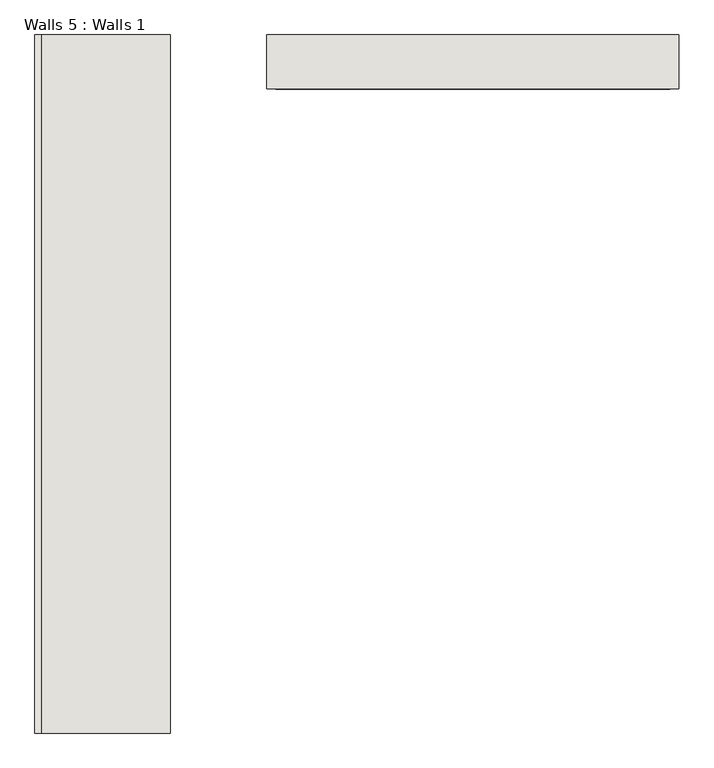
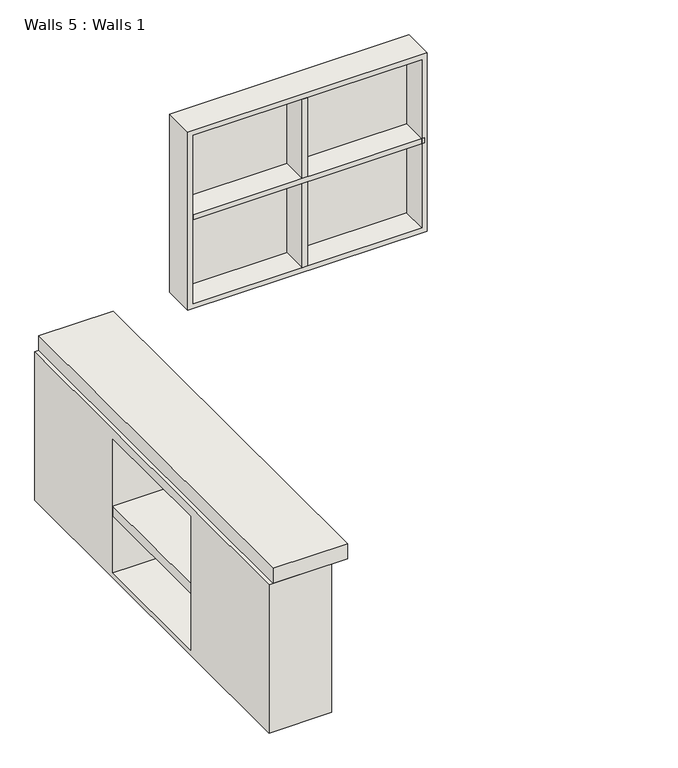
"""IFC4 building model written with IfcOpenShell, lengths in millimetres: wall geometry, Walls 5 : Walls 1."""

from ifc_helpers import new_model, si_unit, frame, origin, place, context, project, spatial, polyline, outline, extrude, faceted_brep, source, transform, mapped, element, save


def walls_5_walls_1_1b2d60d9(model_context):
    return source(origin(), model_context, "Body", "SolidModel", [
        extrude(outline(polyline([(-4669.7681702, -2647.557676), (-4669.7681702, -2774.557676), (-5793.7181702, -2774.557676), (-5793.7181702, -2647.557676), (-4669.7681702, -2647.557676)])), frame((0.0, 0.0, 7723.2031259), z_axis=(0.0, 0.0, 1.0), x_axis=(1.0, 0.0, 0.0)), (0.0, 0.0, 1.0), 25.4),
        extrude(outline(polyline([(-5263.4931702, -2774.557676), (-5263.4931702, -2647.557676), (-5238.0931702, -2647.557676), (-5238.0931702, -2774.557676), (-5263.4931702, -2774.557676)])), frame((0.0, 0.0, 7291.4031259), z_axis=(0.0, 0.0, 1.0), x_axis=(1.0, 0.0, 0.0)), (0.0, 0.0, 1.0), 863.6),
        faceted_brep([(-4657.0681702, -2774.557676, 7266.0031259), (-4657.0681702, -2774.557676, 8180.4031259), (-5819.1181702, -2774.557676, 8180.4031259), (-5819.1181702, -2774.557676, 7266.0031259), (-4682.4681702, -2774.557676, 8155.0031259), (-4682.4681702, -2774.557676, 7291.4031259), (-5793.7181702, -2774.557676, 7291.4031259), (-5793.7181702, -2774.557676, 8155.0031259), (-4657.0681702, -2622.157676, 7266.0031259), (-5819.1181702, -2622.157676, 7266.0031259), (-5819.1181702, -2622.157676, 8180.4031259), (-4657.0681702, -2622.157676, 8180.4031259), (-4682.4681702, -2647.557676, 8155.0031259), (-5793.7181702, -2647.557676, 8155.0031259), (-5793.7181702, -2647.557676, 7291.4031259), (-4682.4681702, -2647.557676, 7291.4031259)], [[[0, 1, 2, 3], [4, 5, 6, 7]], [[8, 9, 10, 11]], [[1, 0, 8, 11]], [[2, 1, 11, 10]], [[3, 2, 10, 9]], [[0, 3, 9, 8]], [[12, 13, 14, 15]], [[12, 15, 5, 4]], [[15, 14, 6, 5]], [[14, 13, 7, 6]], [[13, 12, 4, 7]]]),
        extrude(outline(polyline([(-6454.1181702, -2622.157676), (-6092.1681702, -2622.157676), (-6092.1681702, -4590.657676), (-6454.1181702, -4590.657676), (-6454.1181702, -2622.157676)])), frame((0.0, 0.0, 7189.8031259), z_axis=(0.0, 0.0, 1.0), x_axis=(1.0, 0.0, 0.0)), (0.0, 0.0, 1.0), 76.2),
        extrude(outline(polyline([(-6165.8877015, -3282.4431283), (-6165.8877015, -3592.120176), (-6170.9478577, -3592.120176), (-6170.9478577, -3282.4431283), (-6165.8877015, -3282.4431283)])), frame((0.0, 0.0, 6446.3519176), z_axis=(0.0, 0.0, 1.0), x_axis=(1.0, 0.0, 0.0)), (0.0, 0.0, 1.0), 685.8),
        extrude(outline(polyline([(-6163.308014, -3603.6829064), (-6163.308014, -3930.257676), (-6168.3681702, -3930.257676), (-6168.3681702, -3603.6829064), (-6163.308014, -3603.6829064)])), frame((0.0, 0.0, 6453.2031259), z_axis=(0.0, 0.0, 1.0), x_axis=(1.0, 0.0, 0.0)), (0.0, 0.0, 1.0), 685.8),
        extrude(outline(polyline([(-6168.3681702, -3277.1081367), (-6168.3681702, -3930.257676), (-6473.1681702, -3930.257676), (-6473.1681702, -3277.1081367), (-6168.3681702, -3277.1081367)])), frame((0.0, 0.0, 6745.3031259), z_axis=(0.0, 0.0, 1.0), x_axis=(1.0, 0.0, 0.0)), (0.0, 0.0, 1.0), 50.8),
        extrude(outline(polyline([(-2622.157676, 6427.8031259), (-4590.657676, 6427.8031259), (-4590.657676, 7189.8031259), (-2622.157676, 7189.8031259), (-2622.157676, 6427.8031259)]), holes=[polyline([(-3277.1081367, 6453.2031259), (-3277.1081367, 7139.0031259), (-3930.257676, 7139.0031259), (-3930.257676, 6453.2031259), (-3277.1081367, 6453.2031259)])]), frame((-6473.1681702, 0.0, 0.0), z_axis=(1.0, 0.0, 0.0), x_axis=(0.0, 1.0, 0.0)), (0.0, 0.0, 1.0), 304.8),
        extrude(outline(polyline([(-6165.7884827, -2647.557676), (-6165.7884827, -3257.157676), (-6168.3681702, -3257.157676), (-6168.3681702, -2647.557676), (-6165.7884827, -2647.557676)])), frame((0.0, 0.0, 6456.3781259), z_axis=(0.0, 0.0, 1.0), x_axis=(1.0, 0.0, 0.0)), (0.0, 0.0, 1.0), 298.45),
        extrude(outline(polyline([(-6165.7884827, -2647.557676), (-6165.7884827, -3257.157676), (-6168.3681702, -3257.157676), (-6168.3681702, -2647.557676), (-6165.7884827, -2647.557676)])), frame((0.0, 0.0, 6798.6431259), z_axis=(0.0, 0.0, 1.0), x_axis=(1.0, 0.0, 0.0)), (0.0, 0.0, 1.0), 365.76),
        extrude(outline(polyline([(-6165.7884827, -3955.657676), (-6165.7884827, -4565.257676), (-6168.3681702, -4565.257676), (-6168.3681702, -3955.657676), (-6165.7884827, -3955.657676)])), frame((0.0, 0.0, 6456.3781259), z_axis=(0.0, 0.0, 1.0), x_axis=(1.0, 0.0, 0.0)), (0.0, 0.0, 1.0), 298.45),
        extrude(outline(polyline([(-6165.7884827, -3955.657676), (-6165.7884827, -4565.257676), (-6168.3681702, -4565.257676), (-6168.3681702, -3955.657676), (-6165.7884827, -3955.657676)])), frame((0.0, 0.0, 6798.6431259), z_axis=(0.0, 0.0, 1.0), x_axis=(1.0, 0.0, 0.0)), (0.0, 0.0, 1.0), 365.76),
    ])


if __name__ == "__main__":
    model = new_model("IFC4")
    model_context = context("Model", 3, world=origin())
    ifc_project = project(units=[si_unit("LENGTHUNIT", "METRE", prefix="MILLI")], contexts=[model_context])
    site = spatial("IfcSite", under=ifc_project)
    building = spatial("IfcBuilding", under=site)
    placement = place(None, origin())
    walls_5_walls_1_shape = walls_5_walls_1_1b2d60d9(model_context)
    element("IfcWall", 1, ObjectType="Walls 5 : Walls 1", at=placement, inside=building, context=model_context, shape_type="MappedRepresentation", body=[
        mapped(walls_5_walls_1_shape, transform((0.0, 0.0, 0.0), x_axis=(1.0, 0.0, 0.0), y_axis=(0.0, 1.0, 0.0), z_axis=(0.0, 0.0, 1.0))),
    ])
    save(model, "model.ifc")

# Revit data of these elements
# Element 1 (IfcWall, "Walls 5 : Walls 1")
#   Materials on its faces: "drawers", "wood", "clear glass", "stone", "Default Wall"
# Materials
#   "drawers": class "Generic", colour RGB 121 66 39, transparency 0, Cost = 0
#   "wood": class "Generic", colour RGB 255 226 181, transparency 0, Cost = 0
#   "clear glass": class "Generic", colour RGB 141 181 235, transparency 0.9, Cost = 0
#   "stone": class "Generic", colour RGB 125 126 130, transparency 0, Cost = 0
#   "Default Wall": colour RGB 128 128 128, transparency 0
